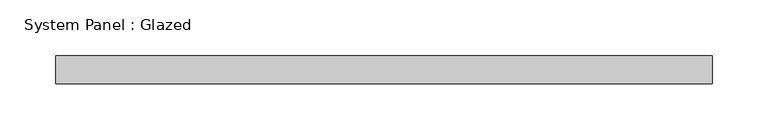
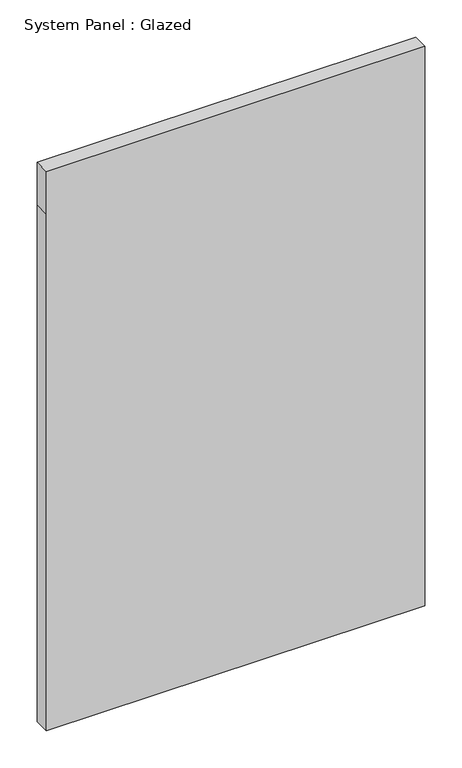
"""IFC4 building model written with IfcOpenShell, lengths in millimetres: plate geometry, System Panel : Glazed."""

from ifc_helpers import new_model, si_unit, frame, origin, place, context, project, spatial, polyline, outline, extrude, source, transform, mapped, element, save


def system_panel_glazed_0c2a6c90(model_context):
    return source(origin(), model_context, "Body", "SweptSolid", [
        extrude(outline(polyline([(0.0, -295.275), (0.0, 295.275), (852.6761324, 295.275), (922.5261324, 295.275), (922.5261324, -295.275), (852.6761324, -295.275), (0.0, -295.275)])), frame((0.0, 19.05, 0.0), z_axis=(0.0, 1.0, 0.0), x_axis=(0.0, 0.0, 1.0)), (0.0, 0.0, 1.0), 25.4),
    ])


if __name__ == "__main__":
    model = new_model("IFC4")
    model_context = context("Model", 3, world=origin())
    ifc_project = project(units=[si_unit("LENGTHUNIT", "METRE", prefix="MILLI")], contexts=[model_context])
    site = spatial("IfcSite", under=ifc_project)
    building = spatial("IfcBuilding", under=site)
    placement = place(None, origin())
    system_panel_glazed_shape = system_panel_glazed_0c2a6c90(model_context)
    element("IfcPlate", 1, ObjectType="System Panel : Glazed", at=placement, inside=building, context=model_context, shape_type="MappedRepresentation", body=[
        mapped(system_panel_glazed_shape, transform((0.0, 0.0, 0.0), x_axis=(1.0, 0.0, 0.0), y_axis=(0.0, 1.0, 0.0), z_axis=(0.0, 0.0, 1.0))),
    ])
    save(model, "model.ifc")

# Revit data of these elements
# Type "System Panel : Glazed"
#   Construction Type Id = "GSP4R"
#   Analytic Construction = "1/8 in Pilkington single glazing"
#   Visual Light Transmittance = 0.9
#   Solar Heat Gain Coefficient = 0.86
#   Heat Transfer Coefficient (U) = 1.18115 BTU/(h·ft²·°F)
#   Define Thermal Properties by = 1
# Element 1 (IfcPlate, "System Panel : Glazed")
#   Materials on its faces: "Glass"
# Materials
#   "Glass": class "Glass", colour RGB 0 128 192, transparency 0.75, Description = "Soda Lime Glass", Cost = 0
